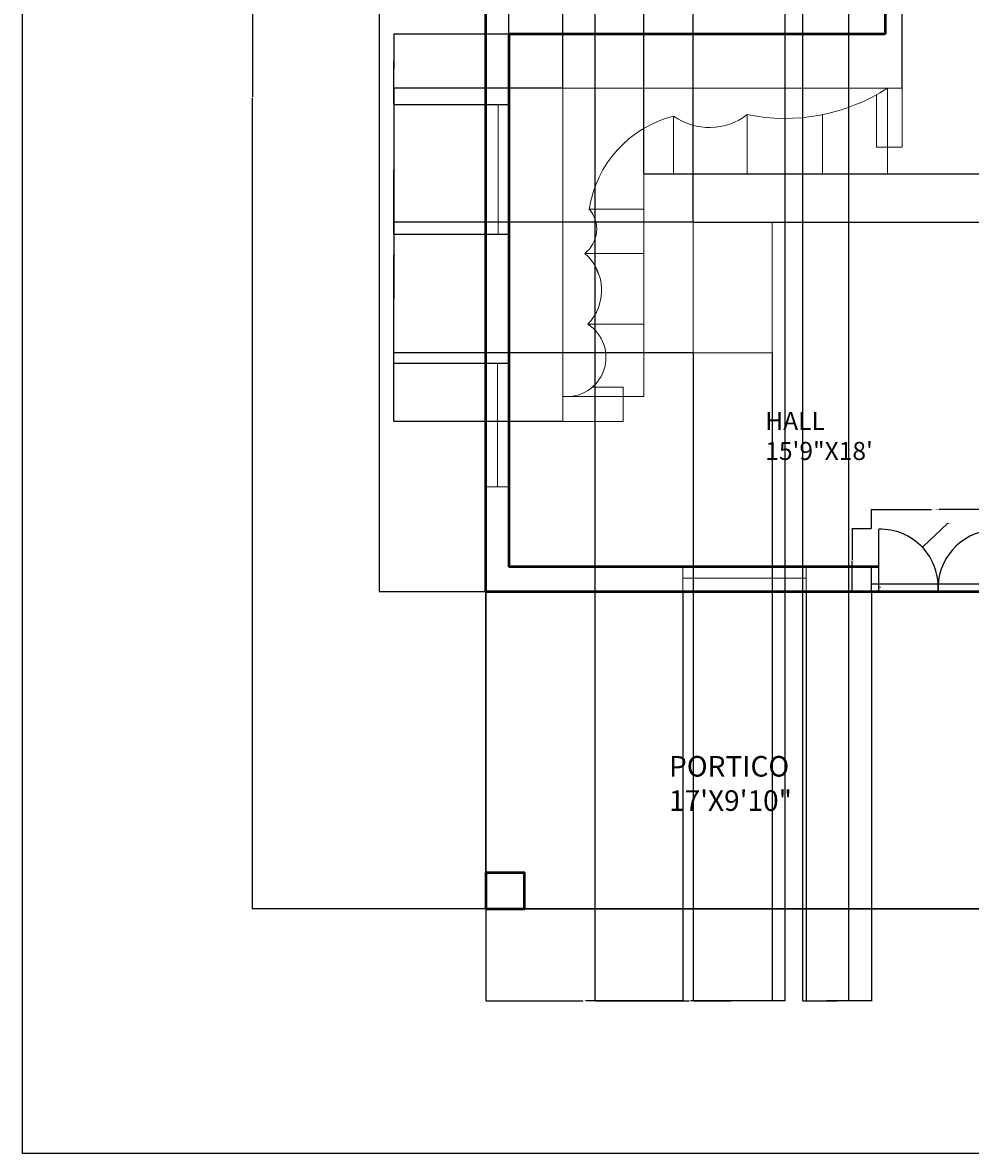
# Model space of a CAD drawing. Units: inches. Extents: x -177 to 2564, y -706 to 2548.
# Tile 1 of 4: x -177 to 192, y -706 to -266. Entities that reach past the tile are written whole.
import ezdxf

# ---------------------------------------------------------------- set-up
doc = ezdxf.new("R2010")
doc.units = ezdxf.units.IN
doc.header["$MEASUREMENT"] = 0
for name, color, linetype, lineweight in [('A-ANNO-DIMS', 2, 'Continuous', 18), ('A-ANNO-TTLB', 7, 'Continuous', 25), ('A-AREA-IDEN', 7, 'Continuous', 25), ('A-COLS', 7, 'Continuous', 50), ('A-DOOR', 3, 'Continuous', 25), ('A-FLOR-OTLN', 7, 'Continuous', 30), ('A-FURN', 8, 'Continuous', 18), ('A-GLAZ', 4, 'Continuous', 18), ('A-WALL', 7, 'Continuous', 50)]:
    doc.layers.add(name, color=color, linetype=linetype, lineweight=lineweight)
doc.styles.get("Standard").update_dxf_attribs({"font": 'arial.ttf'})
doc.dimstyles.get("Standard").update_dxf_attribs({"dimtxt": 0.18, "dimasz": 0.18, "dimexe": 0.18, "dimexo": 0.0625, "dimgap": 0.09, "dimtad": 0, "dimtih": 1, "dimtoh": 1, "dimdec": 0, "dimzin": 0, "dimdsep": 46, "dimlunit": 4, "dimtxsty": 'Standard', "dimcen": 0.09, "dimadec": 0, "dimazin": 0, "dimtfac": 1, "dimtdec": 0, "dimtofl": 0, "dimtmove": 0, "dimatfit": 3, "dimfxl": 1, "dimtolj": 1, "dimtzin": 0, "dimarcsym": 0})

# ---------------------------------------------------------------- blocks, each defined once
blk = doc.blocks.new('*D2')
at = {"layer": 'A-ANNO-DIMS', "color": 0, "lineweight": -2, "transparency": 16777216}
for p, q in [((3.41, 20.54), (-38, 20.54)), ((-37.82, 20.36), (-37.82, -233.15)), ((-37.82, -487.01), (-37.82, -233.51)), ((3.41, -487.19), (-38, -487.19))]:
    blk.add_line(p, q, dxfattribs=at)
at = {"layer": 'A-ANNO-DIMS', "color": 0, "transparency": 16777216}
for points in [[(-37.85, 20.36), (-37.79, 20.36), (-37.82, 20.54)], [(-37.85, -487.01), (-37.79, -487.01), (-37.82, -487.19)]]:
    blk.add_solid(points, dxfattribs=at)
at = {"layer": 'Defpoints', "color": 0, "transparency": 16777216}
for p in [(3.47, 20.54), (-37.82, -487.19), (3.47, -487.19)]:
    blk.add_point(p, dxfattribs=at)
at = {"layer": 'A-ANNO-DIMS', "color": 0, "transparency": 16777216, "insert": (-37.82, -233.33), "char_height": 0.18, "attachment_point": 5}
blk.add_mtext('\\A1;42\'-4"', dxfattribs=at)
blk = doc.blocks.new('*D3')
at = {"layer": 'A-ANNO-DIMS', "color": 0, "lineweight": -2, "transparency": 16777216}
for p, q in [((3.41, 20.54), (-87.46, 20.54)), ((-87.28, 20.36), (-87.28, -294.78)), ((-87.28, -610.28), (-87.28, -295.15)), ((3.41, -610.46), (-87.46, -610.46))]:
    blk.add_line(p, q, dxfattribs=at)
at = {"layer": 'A-ANNO-DIMS', "color": 0, "transparency": 16777216}
for points in [[(-87.31, 20.36), (-87.25, 20.36), (-87.28, 20.54)], [(-87.31, -610.28), (-87.25, -610.28), (-87.28, -610.46)]]:
    blk.add_solid(points, dxfattribs=at)
at = {"layer": 'Defpoints', "color": 0, "transparency": 16777216}
for p in [(3.47, 20.54), (-87.28, -610.46), (3.47, -610.46)]:
    blk.add_point(p, dxfattribs=at)
at = {"layer": 'A-ANNO-DIMS', "color": 0, "transparency": 16777216, "insert": (-87.28, -294.96), "char_height": 0.18, "attachment_point": 5}
blk.add_mtext('\\A1;52\'-7"', dxfattribs=at)
blk = doc.blocks.new('WIN-48')
for p, q in [((0, 0), (9, 0)), ((9, 0), (4.59, 0)), ((4.59, 0), (4.59, -48.06)), ((9, -48.06), (0, -48.06))]:
    blk.add_line(p, q)
blk = doc.blocks.new('DOOR-PAIR-44')
for p, q in [((0, 0), (0, 24.32)), ((44.01, 0), (44.01, 23.95)), ((-2.88, 0), (-2.88, 3.11)), ((-2.88, 3.11), (46.72, 3.11)), ((46.72, 0), (-2.88, 0)), ((-2.88, 0), (0, 0)), ((0, 0), (44.01, 0)), ((23.01, 0), (23.01, 3.55)), ((44.01, 0), (23.01, 0)), ((46.72, 0), (44.01, 0))]:
    blk.add_line(p, q)
for centre, radius, start, end in [((0.52, 1.77), 22.55, 355.4915, 91.326), ((45.7, 1.28), 22.73, 94.2755, 183.2347)]:
    blk.add_arc(centre, radius, start, end)
blk = doc.blocks.new('*D20')
at = {"layer": 'A-ANNO-DIMS', "color": 0, "lineweight": -2, "transparency": 16777216}
for p, q in [((153.41, -462.66), (153.41, -455.1)), ((153.59, -455.28), (176.76, -455.28)), ((202.83, -455.28), (179.66, -455.28)), ((203.01, -462.66), (203.01, -455.1))]:
    blk.add_line(p, q, dxfattribs=at)
at = {"layer": 'A-ANNO-DIMS', "color": 0, "transparency": 16777216}
for points in [[(153.59, -455.25), (153.59, -455.31), (153.41, -455.28)], [(202.83, -455.25), (202.83, -455.31), (203.01, -455.28)]]:
    blk.add_solid(points, dxfattribs=at)
at = {"layer": 'Defpoints', "color": 0, "transparency": 16777216}
for p in [(203.01, -455.28), (153.41, -462.72), (203.01, -462.72)]:
    blk.add_point(p, dxfattribs=at)
at = {"layer": 'A-ANNO-DIMS', "color": 0, "transparency": 16777216, "insert": (178.21, -455.28), "char_height": 0.18, "attachment_point": 5}
blk.add_mtext('\\A1;DOOR D3 4\'-1 1/2" TYP.', dxfattribs=at)
blk = doc.blocks.new('*D21')
at = {"layer": 'A-ANNO-DIMS', "color": 0, "lineweight": -2, "transparency": 16777216}
for p, q in [((153.34, -462.72), (145.79, -462.72)), ((145.97, -462.9), (145.97, -474.77)), ((145.97, -487.01), (145.97, -475.14)), ((153.34, -487.19), (145.79, -487.19))]:
    blk.add_line(p, q, dxfattribs=at)
at = {"layer": 'A-ANNO-DIMS', "color": 0, "transparency": 16777216}
for points in [[(145.94, -462.9), (146, -462.9), (145.97, -462.72)], [(145.94, -487.01), (146, -487.01), (145.97, -487.19)]]:
    blk.add_solid(points, dxfattribs=at)
at = {"layer": 'Defpoints', "color": 0, "transparency": 16777216}
for p in [(145.97, -462.72), (153.41, -462.72), (153.41, -487.19)]:
    blk.add_point(p, dxfattribs=at)
at = {"layer": 'A-ANNO-DIMS', "color": 0, "transparency": 16777216, "insert": (145.97, -474.95), "char_height": 0.18, "attachment_point": 5}
blk.add_mtext('\\A1;2\'-0 1/2" TYP.', dxfattribs=at)
blk = doc.blocks.new('*D22')
at = {"layer": 'A-ANNO-DIMS', "color": 0, "lineweight": -2, "transparency": 16777216}
for p, q in [((33.37, -291.35), (33.37, 71.74)), ((33.55, 71.56), (98.96, 71.56)), ((165.15, 71.56), (99.74, 71.56)), ((165.33, -291.35), (165.33, 71.74))]:
    blk.add_line(p, q, dxfattribs=at)
at = {"layer": 'A-ANNO-DIMS', "color": 0, "transparency": 16777216}
for points in [[(33.55, 71.59), (33.55, 71.53), (33.37, 71.56)], [(165.15, 71.59), (165.15, 71.53), (165.33, 71.56)]]:
    blk.add_solid(points, dxfattribs=at)
at = {"layer": 'Defpoints', "color": 0, "transparency": 16777216}
for p in [(165.33, 71.56), (33.37, -291.42), (165.33, -291.42)]:
    blk.add_point(p, dxfattribs=at)
at = {"layer": 'A-ANNO-DIMS', "color": 0, "transparency": 16777216, "insert": (99.35, 71.56), "char_height": 0.18, "attachment_point": 5}
blk.add_mtext('\\A1;11\'-0"', dxfattribs=at)
blk = doc.blocks.new('*D23')
at = {"layer": 'A-ANNO-DIMS', "color": 0, "lineweight": -2, "transparency": 16777216}
for p, q in [((33.31, -291.42), (-32.41, -291.42)), ((-32.23, -291.6), (-32.23, -356.01)), ((-32.23, -420.78), (-32.23, -356.37)), ((33.31, -420.96), (-32.41, -420.96))]:
    blk.add_line(p, q, dxfattribs=at)
at = {"layer": 'A-ANNO-DIMS', "color": 0, "transparency": 16777216}
for points in [[(-32.26, -291.6), (-32.2, -291.6), (-32.23, -291.42)], [(-32.26, -420.78), (-32.2, -420.78), (-32.23, -420.96)]]:
    blk.add_solid(points, dxfattribs=at)
at = {"layer": 'Defpoints', "color": 0, "transparency": 16777216}
for p in [(33.37, -291.42), (-32.23, -420.96), (33.37, -420.96)]:
    blk.add_point(p, dxfattribs=at)
at = {"layer": 'A-ANNO-DIMS', "color": 0, "transparency": 16777216, "insert": (-32.23, -356.19), "char_height": 0.18, "attachment_point": 5}
blk.add_mtext('\\A1;10\'-9 1/2"', dxfattribs=at)
blk = doc.blocks.new('*D24')
at = {"layer": 'A-ANNO-DIMS', "color": 0, "lineweight": -2, "transparency": 16777216}
for p, q in [((84.06, -394.33), (84.06, -646.34)), ((114.78, -394.33), (114.78, -646.34)), ((84.24, -646.16), (98.88, -646.16)), ((114.6, -646.16), (99.96, -646.16))]:
    blk.add_line(p, q, dxfattribs=at)
at = {"layer": 'A-ANNO-DIMS', "color": 0, "transparency": 16777216}
for points in [[(84.24, -646.13), (84.24, -646.19), (84.06, -646.16)], [(114.6, -646.13), (114.6, -646.19), (114.78, -646.16)]]:
    blk.add_solid(points, dxfattribs=at)
at = {"layer": 'Defpoints', "color": 0, "transparency": 16777216}
for p in [(84.06, -394.27), (114.78, -394.27), (114.78, -646.16)]:
    blk.add_point(p, dxfattribs=at)
at = {"layer": 'A-ANNO-DIMS', "color": 0, "transparency": 16777216, "insert": (99.42, -646.16), "char_height": 0.18, "attachment_point": 5}
blk.add_mtext('\\A1;2\'-6 1/2"', dxfattribs=at)
blk = doc.blocks.new('*D25')
at = {"layer": 'A-ANNO-DIMS', "color": 0, "lineweight": -2, "transparency": 16777216}
for p, q in [((84, -343.5), (-32.41, -343.5)), ((-32.23, -343.68), (-32.23, -368.7)), ((-32.23, -394.09), (-32.23, -369.07)), ((84, -394.27), (-32.41, -394.27))]:
    blk.add_line(p, q, dxfattribs=at)
at = {"layer": 'A-ANNO-DIMS', "color": 0, "transparency": 16777216}
for points in [[(-32.26, -343.68), (-32.2, -343.68), (-32.23, -343.5)], [(-32.26, -394.09), (-32.2, -394.09), (-32.23, -394.27)]]:
    blk.add_solid(points, dxfattribs=at)
at = {"layer": 'Defpoints', "color": 0, "transparency": 16777216}
for p in [(-32.23, -343.5), (84.06, -343.5), (84.06, -394.27)]:
    blk.add_point(p, dxfattribs=at)
at = {"layer": 'A-ANNO-DIMS', "color": 0, "transparency": 16777216, "insert": (-32.23, -368.89), "char_height": 0.18, "attachment_point": 5}
blk.add_mtext('\\A1;4\'-3"', dxfattribs=at)
blk = doc.blocks.new('*D26')
at = {"layer": 'A-ANNO-DIMS', "color": 0, "lineweight": -2, "transparency": 16777216}
for p, q in [((64.94, -324.62), (64.94, 71.74)), ((65.12, 71.56), (74.18, 71.56)), ((83.88, 71.56), (74.82, 71.56)), ((84.06, -343.44), (84.06, 71.74))]:
    blk.add_line(p, q, dxfattribs=at)
at = {"layer": 'A-ANNO-DIMS', "color": 0, "transparency": 16777216}
for points in [[(65.12, 71.59), (65.12, 71.53), (64.94, 71.56)], [(83.88, 71.59), (83.88, 71.53), (84.06, 71.56)]]:
    blk.add_solid(points, dxfattribs=at)
at = {"layer": 'Defpoints', "color": 0, "transparency": 16777216}
for p in [(84.06, 71.56), (64.94, -324.69), (84.06, -343.5)]:
    blk.add_point(p, dxfattribs=at)
at = {"layer": 'A-ANNO-DIMS', "color": 0, "transparency": 16777216, "insert": (74.5, 71.56), "char_height": 0.18, "attachment_point": 5}
blk.add_mtext('\\A1;1\'-7"', dxfattribs=at)
blk = doc.blocks.new('*D27')
at = {"layer": 'A-ANNO-DIMS', "color": 0, "lineweight": -2, "transparency": 16777216}
for p, q in [((65.01, -324.69), (417.35, -324.69)), ((417.17, -324.87), (417.17, -333.91)), ((417.17, -343.32), (417.17, -334.27)), ((84.12, -343.5), (417.35, -343.5))]:
    blk.add_line(p, q, dxfattribs=at)
at = {"layer": 'A-ANNO-DIMS', "color": 0, "transparency": 16777216}
for points in [[(417.14, -324.87), (417.2, -324.87), (417.17, -324.69)], [(417.14, -343.32), (417.2, -343.32), (417.17, -343.5)]]:
    blk.add_solid(points, dxfattribs=at)
at = {"layer": 'Defpoints', "color": 0, "transparency": 16777216}
for p in [(64.94, -324.69), (84.06, -343.5), (417.17, -343.5)]:
    blk.add_point(p, dxfattribs=at)
at = {"layer": 'A-ANNO-DIMS', "color": 0, "transparency": 16777216, "insert": (417.17, -334.09), "char_height": 0.18, "attachment_point": 5}
blk.add_mtext('\\A1;1\'-7"', dxfattribs=at)
blk = doc.blocks.new('*D28')
at = {"layer": 'A-ANNO-DIMS', "color": 0, "lineweight": -2, "transparency": 16777216}
for p, q in [((12.47, -270.4), (12.47, 71.74)), ((12.65, 71.56), (22.6, 71.56)), ((33.19, 71.56), (23.24, 71.56)), ((33.37, -291.35), (33.37, 71.74))]:
    blk.add_line(p, q, dxfattribs=at)
at = {"layer": 'A-ANNO-DIMS', "color": 0, "transparency": 16777216}
for points in [[(12.65, 71.59), (12.65, 71.53), (12.47, 71.56)], [(33.19, 71.59), (33.19, 71.53), (33.37, 71.56)]]:
    blk.add_solid(points, dxfattribs=at)
at = {"layer": 'Defpoints', "color": 0, "transparency": 16777216}
for p in [(33.37, 71.56), (12.47, -270.46), (33.37, -291.42)]:
    blk.add_point(p, dxfattribs=at)
at = {"layer": 'A-ANNO-DIMS', "color": 0, "transparency": 16777216, "insert": (22.92, 71.56), "char_height": 0.18, "attachment_point": 5}
blk.add_mtext('\\A1;1\'-9"', dxfattribs=at)
blk = doc.blocks.new('*D29')
at = {"layer": 'A-ANNO-DIMS', "color": 0, "lineweight": -2, "transparency": 16777216}
for p, q in [((12.41, -270.46), (-32.41, -270.46)), ((-32.23, -270.64), (-32.23, -280.76)), ((-32.23, -291.24), (-32.23, -281.12)), ((33.31, -291.42), (-32.41, -291.42))]:
    blk.add_line(p, q, dxfattribs=at)
at = {"layer": 'A-ANNO-DIMS', "color": 0, "transparency": 16777216}
for points in [[(-32.26, -270.64), (-32.2, -270.64), (-32.23, -270.46)], [(-32.26, -291.24), (-32.2, -291.24), (-32.23, -291.42)]]:
    blk.add_solid(points, dxfattribs=at)
at = {"layer": 'Defpoints', "color": 0, "transparency": 16777216}
for p in [(12.47, -270.46), (-32.23, -291.42), (33.37, -291.42)]:
    blk.add_point(p, dxfattribs=at)
at = {"layer": 'A-ANNO-DIMS', "color": 0, "transparency": 16777216, "insert": (-32.23, -280.94), "char_height": 0.18, "attachment_point": 5}
blk.add_mtext('\\A1;1\'-9"', dxfattribs=at)
blk = doc.blocks.new('*D32')
at = {"layer": 'A-ANNO-DIMS', "color": 0, "lineweight": -2, "transparency": 16777216}
for p, q in [((45.91, -17.28), (45.91, -646.34)), ((119.76, -17.28), (119.76, -646.34)), ((46.09, -646.16), (82.5, -646.16)), ((119.58, -646.16), (83.16, -646.16))]:
    blk.add_line(p, q, dxfattribs=at)
at = {"layer": 'A-ANNO-DIMS', "color": 0, "transparency": 16777216}
for points in [[(46.09, -646.13), (46.09, -646.19), (45.91, -646.16)], [(119.58, -646.13), (119.58, -646.19), (119.76, -646.16)]]:
    blk.add_solid(points, dxfattribs=at)
at = {"layer": 'Defpoints', "color": 0, "transparency": 16777216}
for p in [(45.91, -17.21), (119.76, -17.21), (119.76, -646.16)]:
    blk.add_point(p, dxfattribs=at)
at = {"layer": 'A-ANNO-DIMS', "color": 0, "transparency": 16777216, "insert": (82.83, -646.16), "char_height": 0.18, "attachment_point": 5}
blk.add_mtext('\\A1;6\'-2"', dxfattribs=at)
blk = doc.blocks.new('*D33')
at = {"layer": 'A-ANNO-DIMS', "color": 0, "lineweight": -2, "transparency": 16777216}
for p, q in [((126.64, -61.62), (126.64, -646.34)), ((144.47, -61.62), (144.47, -646.34)), ((126.82, -646.16), (135.24, -646.16)), ((144.29, -646.16), (135.88, -646.16))]:
    blk.add_line(p, q, dxfattribs=at)
at = {"layer": 'A-ANNO-DIMS', "color": 0, "transparency": 16777216}
for points in [[(126.82, -646.13), (126.82, -646.19), (126.64, -646.16)], [(144.29, -646.13), (144.29, -646.19), (144.47, -646.16)]]:
    blk.add_solid(points, dxfattribs=at)
at = {"layer": 'Defpoints', "color": 0, "transparency": 16777216}
for p in [(126.64, -61.56), (144.47, -61.56), (144.47, -646.16)]:
    blk.add_point(p, dxfattribs=at)
at = {"layer": 'A-ANNO-DIMS', "color": 0, "transparency": 16777216, "insert": (135.56, -646.16), "char_height": 0.18, "attachment_point": 5}
blk.add_mtext('\\A1;1\'-6"', dxfattribs=at)
blk = doc.blocks.new('*D38')
at = {"layer": 'A-ANNO-DIMS', "color": 0, "lineweight": -2, "transparency": 16777216}
for p, q in [((3.47, -487.25), (3.47, -646.34)), ((80.08, -487.25), (80.08, -646.34)), ((3.65, -646.16), (41.24, -646.16)), ((79.9, -646.16), (42.32, -646.16))]:
    blk.add_line(p, q, dxfattribs=at)
at = {"layer": 'A-ANNO-DIMS', "color": 0, "transparency": 16777216}
for points in [[(3.65, -646.13), (3.65, -646.19), (3.47, -646.16)], [(79.9, -646.13), (79.9, -646.19), (80.08, -646.16)]]:
    blk.add_solid(points, dxfattribs=at)
at = {"layer": 'Defpoints', "color": 0, "transparency": 16777216}
for p in [(3.47, -487.19), (80.08, -487.19), (80.08, -646.16)]:
    blk.add_point(p, dxfattribs=at)
at = {"layer": 'A-ANNO-DIMS', "color": 0, "transparency": 16777216, "insert": (41.78, -646.16), "char_height": 0.18, "attachment_point": 5}
blk.add_mtext('\\A1;6\'-4 1/2"', dxfattribs=at)
blk = doc.blocks.new('*D39')
at = {"layer": 'A-ANNO-DIMS', "color": 0, "lineweight": -2, "transparency": 16777216}
for p, q in [((128.08, -487.25), (128.08, -646.34)), ((153.41, -487.25), (153.41, -646.34)), ((128.26, -646.16), (140.2, -646.16)), ((153.23, -646.16), (141.28, -646.16))]:
    blk.add_line(p, q, dxfattribs=at)
at = {"layer": 'A-ANNO-DIMS', "color": 0, "transparency": 16777216}
for points in [[(128.26, -646.13), (128.26, -646.19), (128.08, -646.16)], [(153.23, -646.13), (153.23, -646.19), (153.41, -646.16)]]:
    blk.add_solid(points, dxfattribs=at)
at = {"layer": 'Defpoints', "color": 0, "transparency": 16777216}
for p in [(128.08, -487.19), (153.41, -487.19), (153.41, -646.16)]:
    blk.add_point(p, dxfattribs=at)
at = {"layer": 'A-ANNO-DIMS', "color": 0, "transparency": 16777216, "insert": (140.74, -646.16), "char_height": 0.18, "attachment_point": 5}
blk.add_mtext('\\A1;2\'-1 1/2"', dxfattribs=at)
blk = doc.blocks.new('*D56')
at = {"layer": 'A-ANNO-DIMS', "color": 0, "lineweight": -2, "transparency": 16777216}
for p, q in [((12.41, -270.46), (-32.41, -270.46)), ((-32.23, -270.64), (-32.23, -284)), ((-32.23, -297.73), (-32.23, -284.37)), ((12.41, -297.91), (-32.41, -297.91))]:
    blk.add_line(p, q, dxfattribs=at)
at = {"layer": 'A-ANNO-DIMS', "color": 0, "transparency": 16777216}
for points in [[(-32.26, -270.64), (-32.2, -270.64), (-32.23, -270.46)], [(-32.26, -297.73), (-32.2, -297.73), (-32.23, -297.91)]]:
    blk.add_solid(points, dxfattribs=at)
at = {"layer": 'Defpoints', "color": 0, "transparency": 16777216}
for p in [(12.47, -270.46), (-32.23, -297.91), (12.47, -297.91)]:
    blk.add_point(p, dxfattribs=at)
at = {"layer": 'A-ANNO-DIMS', "color": 0, "transparency": 16777216, "insert": (-32.23, -284.19), "char_height": 0.18, "attachment_point": 5}
blk.add_mtext('\\A1;2\'-3 1/2"', dxfattribs=at)
blk = doc.blocks.new('*D57')
at = {"layer": 'A-ANNO-DIMS', "color": 0, "lineweight": -2, "transparency": 16777216}
for p, q in [((12.41, -297.91), (-32.41, -297.91)), ((-32.23, -298.09), (-32.23, -322.91)), ((-32.23, -348.09), (-32.23, -323.27)), ((12.41, -348.27), (-32.41, -348.27))]:
    blk.add_line(p, q, dxfattribs=at)
at = {"layer": 'A-ANNO-DIMS', "color": 0, "transparency": 16777216}
for points in [[(-32.26, -298.09), (-32.2, -298.09), (-32.23, -297.91)], [(-32.26, -348.09), (-32.2, -348.09), (-32.23, -348.27)]]:
    blk.add_solid(points, dxfattribs=at)
at = {"layer": 'Defpoints', "color": 0, "transparency": 16777216}
for p in [(12.47, -297.91), (-32.23, -348.27), (12.47, -348.27)]:
    blk.add_point(p, dxfattribs=at)
at = {"layer": 'A-ANNO-DIMS', "color": 0, "transparency": 16777216, "insert": (-32.23, -323.09), "char_height": 0.18, "attachment_point": 5}
blk.add_mtext('\\A1;4\'-2 1/2"', dxfattribs=at)
blk = doc.blocks.new('*D58')
at = {"layer": 'A-ANNO-DIMS', "color": 0, "lineweight": -2, "transparency": 16777216}
for p, q in [((12.41, -348.27), (-32.41, -348.27)), ((-32.23, -348.45), (-32.23, -373.16)), ((-32.23, -398.23), (-32.23, -373.52)), ((12.41, -398.41), (-32.41, -398.41))]:
    blk.add_line(p, q, dxfattribs=at)
at = {"layer": 'A-ANNO-DIMS', "color": 0, "transparency": 16777216}
for points in [[(-32.26, -348.45), (-32.2, -348.45), (-32.23, -348.27)], [(-32.26, -398.23), (-32.2, -398.23), (-32.23, -398.41)]]:
    blk.add_solid(points, dxfattribs=at)
at = {"layer": 'Defpoints', "color": 0, "transparency": 16777216}
for p in [(12.47, -348.27), (-32.23, -398.41), (12.47, -398.41)]:
    blk.add_point(p, dxfattribs=at)
at = {"layer": 'A-ANNO-DIMS', "color": 0, "transparency": 16777216, "insert": (-32.23, -373.34), "char_height": 0.18, "attachment_point": 5}
blk.add_mtext('\\A1;4\'-2"', dxfattribs=at)
blk = doc.blocks.new('*D65')
at = {"layer": 'A-ANNO-DIMS', "color": 0, "lineweight": -2, "transparency": 16777216}
for p, q in [((183.03, -460.62), (173.33, -469.79)), ((183.21, -460.62), (183.03, -460.62)), ((156.72, -485.41), (156.9, -485.41)), ((156.81, -485.5), (156.81, -485.32))]:
    blk.add_line(p, q, dxfattribs=at)
at = {"layer": 'A-ANNO-DIMS', "color": 0, "transparency": 16777216}
blk.add_solid([(173.31, -469.77), (173.35, -469.81), (173.2, -469.92)], dxfattribs=at)
at = {"layer": 'Defpoints', "color": 0, "transparency": 16777216}
for p in [(173.2, -469.92), (156.81, -485.41)]:
    blk.add_point(p, dxfattribs=at)
at = {"layer": 'A-ANNO-DIMS', "color": 0, "transparency": 16777216, "insert": (184.1, -460.62), "char_height": 0.18, "attachment_point": 5}
blk.add_mtext('\\A1;2X R1\'-10 1/2"', dxfattribs=at)

msp = doc.modelspace()

# ---------------------------------------------------------------- linework, layer by layer
at = {"layer": 'A-ANNO-TTLB'}
msp.add_lwpolyline([(-176.6, 185.58), (523.32, 185.58), (523.32, -705.52), (-176.6, -705.52)], close=True, dxfattribs=at)
at = {"layer": 'A-COLS'}
msp.add_lwpolyline([(3.47, -610.46), (18.48, -610.46), (18.48, -596.46), (3.47, -596.46)], close=True, dxfattribs=at)
at = {"layer": 'A-DOOR'}
msp.add_line((153.41, -487.19), (153.41, -477.46), dxfattribs=at)
at = {"layer": 'A-FLOR-OTLN'}
for p, q in [((3.47, -601.46), (3.47, -487.19)), ((3.47, -610.46), (3.47, -601.46)), ((228.47, -610.46), (3.47, -610.46))]:
    msp.add_line(p, q, dxfattribs=at)
at = {"layer": 'A-FURN'}
for p, q in [((33.37, -291.42), (159.67, -291.42)), ((33.37, -411.3), (33.37, -291.42)), ((155.39, -314.44), (155.39, -293.99)), ((159.67, -291.42), (159.67, -324.69)), ((159.67, -291.42), (165.33, -291.42)), ((165.33, -291.42), (165.33, -314.44)), ((76.43, -324.69), (76.43, -302.31)), ((105.13, -324.69), (105.13, -301.74)), ((134.41, -324.69), (134.41, -301.74)), ((165.33, -314.44), (155.39, -314.44)), ((159.67, -324.69), (64.94, -324.69)), ((64.94, -324.69), (64.94, -411.3)), ((105.13, -324.69), (76.43, -324.69)), ((134.41, -324.69), (105.13, -324.69)), ((159.67, -324.69), (134.41, -324.69)), ((64.94, -338.45), (43.7, -338.45)), ((64.94, -355.66), (64.94, -338.45)), ((64.94, -355.66), (41.98, -355.66)), ((64.94, -383.2), (64.94, -355.66)), ((64.94, -383.2), (43.13, -383.2)), ((64.94, -411.3), (64.94, -383.2)), ((56.92, -407.71), (44.83, -407.71)), ((56.92, -420.96), (56.92, -407.71)), ((64.94, -411.3), (33.37, -411.3)), ((33.37, -411.3), (33.37, -420.96)), ((33.37, -420.96), (56.92, -420.96))]:
    msp.add_line(p, q, dxfattribs=at)
msp.add_lwpolyline([(84.06, -343.5), (114.78, -343.5), (114.78, -394.27), (84.06, -394.27)], close=True, dxfattribs=at)
for centre, radius, start, end in [((119.77, -229.86), 73.36, 258.488, 302.952), ((87.39, -345.13), 44.19, 104.3618, 171.3148), ((90.39, -282.55), 24.2, 234.764, 307.5256), ((34.63, -346.24), 11.95, 307.9515, 40.6177), ((29.44, -369.98), 19.03, 315.9974, 48.7785), ((87.39, -345.13), 44.19, 200.4463, 205.9744), ((34.89, -396.09), 15.3, 264.277, 57.4256)]:
    msp.add_arc(centre, radius, start, end, dxfattribs=at)
at = {"layer": 'A-GLAZ'}
for p, q in [((12.47, -297.91), (3.47, -297.91)), ((3.47, -297.91), (3.47, -348.27)), ((8.31, -348.27), (8.31, -297.91)), ((3.47, -348.27), (12.47, -348.27)), ((12.47, -348.27), (8.31, -348.27)), ((12.47, -348.27), (12.47, -348.27)), ((3.47, -446.47), (3.47, -398.41)), ((80.08, -487.19), (80.08, -477.46)), ((80.08, -477.46), (80.08, -481.92)), ((128.08, -477.46), (128.08, -487.19)), ((80.08, -481.92), (128.08, -481.92)), ((128.08, -487.19), (80.08, -487.19))]:
    msp.add_line(p, q, dxfattribs=at)
at = {"layer": 'A-WALL'}
for p, q in [((3.47, -483.46), (3.47, 20.54)), ((158.78, -261.46), (158.78, -270.46)), ((158.78, -270.46), (12.47, -270.46)), ((12.47, -270.46), (12.47, -297.91)), ((12.47, -270.46), (12.47, -477.46)), ((156.29, -477.46), (12.47, -477.46)), ((153.41, -477.46), (128.08, -477.46)), ((3.47, -487.19), (3.47, -483.46)), ((219.47, -487.19), (3.47, -487.19))]:
    msp.add_line(p, q, dxfattribs=at)

# ---------------------------------------------------------------- block references
at = {"layer": 'A-DOOR'}
msp.add_blockref('DOOR-PAIR-44', (156.29, -487.19), dxfattribs=at)
at = {"layer": 'A-GLAZ'}
msp.add_blockref('WIN-48', (3.47, -398.41), dxfattribs=at)

# ---------------------------------------------------------------- texts
at = {"layer": 'A-AREA-IDEN', "insert": (112.13, -417.3), "char_height": 7, "attachment_point": 1}
msp.add_mtext_dynamic_manual_height_columns('HALL\\P15\'9"X18\'', width=0.5909, gutter_width=1, heights=[0], dxfattribs=at)
at = {"layer": 'A-AREA-IDEN', "insert": (74.71, -551.05), "char_height": 8, "attachment_point": 1}
msp.add_mtext('PORTICO\\P17\'X9\'10"', dxfattribs=at)

# ---------------------------------------------------------------- dimensions: what is measured, and where the dimension line sits
at = {"layer": 'A-ANNO-DIMS'}
for base, p1, p2, picture, middle in [((33.37, 71.56), (12.47, -270.46), (33.37, -291.42), '*D28', (22.92, 71.56)), ((165.33, 71.56), (33.37, -291.42), (165.33, -291.42), '*D22', (99.35, 71.56)), ((84.06, 71.56), (64.94, -324.69), (84.06, -343.5), '*D26', (74.5, 71.56)), ((119.7563, -646.1645), (45.9113, -17.2143), (119.7563, -17.2143), '*D32', (82.8338, -646.1645)), ((144.47, -646.16), (126.64, -61.56), (144.47, -61.56), '*D33', (135.56, -646.16)), ((114.78, -646.16), (84.06, -394.27), (114.78, -394.27), '*D24', (99.42, -646.16)), ((80.08, -646.16), (3.47, -487.19), (80.08, -487.19), '*D38', (41.78, -646.16)), ((153.41, -646.16), (128.08, -487.19), (153.41, -487.19), '*D39', (140.74, -646.16))]:
    dim = msp.add_linear_dim(base=base, p1=p1, p2=p2, dimstyle='Standard', override={"dimdec": 1, "dimlfac": 1, "dimrnd": 0, "dimzin": 1, "dimdsep": 46, "dimlunit": 4, "dimfrac": 2}, dxfattribs=at)
    dim.commit()
    dim.dimension.update_dxf_attribs({"geometry": picture, "text_midpoint": middle})
for base, p1, p2, override, picture, middle in [((-87.28, -610.46), (3.47, 20.54), (3.47, -610.46), {"dimclrd": 0, "dimclre": 0, "dimclrt": 0}, '*D3', (-87.28, -294.96)), ((-37.82, -487.19), (3.47, 20.54), (3.47, -487.19), {"dimclrd": 0, "dimclre": 0, "dimclrt": 0}, '*D2', (-37.82, -233.33)), ((-32.2267, -297.9061), (12.4733, -270.4645), (12.4733, -297.9061), {"dimdec": 1, "dimlfac": 1, "dimrnd": 0, "dimzin": 1, "dimdsep": 46, "dimlunit": 4, "dimfrac": 2}, '*D56', (-32.2267, -284.1853)), ((-32.23, -291.42), (12.47, -270.46), (33.37, -291.42), {"dimdec": 1, "dimlfac": 1, "dimrnd": 0, "dimzin": 1, "dimdsep": 46, "dimlunit": 4, "dimfrac": 2}, '*D29', (-32.23, -280.94)), ((-32.23, -420.96), (33.37, -291.42), (33.37, -420.96), {"dimdec": 1, "dimlfac": 1, "dimrnd": 0, "dimzin": 1, "dimdsep": 46, "dimlunit": 4, "dimfrac": 2}, '*D23', (-32.23, -356.19)), ((-32.23, -348.27), (12.47, -297.91), (12.47, -348.27), {"dimdec": 1, "dimlfac": 1, "dimrnd": 0, "dimzin": 1, "dimdsep": 46, "dimlunit": 4, "dimfrac": 2}, '*D57', (-32.23, -323.09)), ((417.17, -343.5), (64.94, -324.69), (84.06, -343.5), {"dimdec": 1, "dimlfac": 1, "dimrnd": 0, "dimzin": 1, "dimdsep": 46, "dimlunit": 4, "dimfrac": 2}, '*D27', (417.17, -334.09)), ((-32.23, -343.5), (84.06, -394.27), (84.06, -343.5), {"dimdec": 1, "dimlfac": 1, "dimrnd": 0, "dimzin": 1, "dimdsep": 46, "dimlunit": 4, "dimfrac": 2}, '*D25', (-32.23, -368.89)), ((-32.23, -398.41), (12.47, -348.27), (12.47, -398.41), {"dimdec": 1, "dimlfac": 1, "dimrnd": 0, "dimzin": 1, "dimdsep": 46, "dimlunit": 4, "dimfrac": 2}, '*D58', (-32.23, -373.34))]:
    dim = msp.add_linear_dim(base=base, p1=p1, p2=p2, angle=90, dimstyle='Standard', override=override, dxfattribs=at)
    dim.commit()
    dim.dimension.update_dxf_attribs({"geometry": picture, "text_midpoint": middle})
dim = msp.add_linear_dim(base=(203.01, -455.28), p1=(153.41, -462.72), p2=(203.01, -462.72), text='DOOR D3 <> TYP.', dimstyle='Standard', override={"dimdec": 1, "dimlfac": 1, "dimrnd": 0, "dimzin": 1, "dimdsep": 46, "dimlunit": 4, "dimfrac": 2}, dxfattribs=at)
dim.commit()
dim.dimension.update_dxf_attribs({"geometry": '*D20', "text_midpoint": (178.21, -455.28)})
dim = msp.add_radius_dim(center=(156.81, -485.41), mpoint=(173.2, -469.92), text='2X <>', dimstyle='Standard', override={"dimdec": 1, "dimlfac": 1, "dimrnd": 0, "dimzin": 1, "dimdsep": 46, "dimlunit": 4, "dimfrac": 2}, dxfattribs=at)
dim.commit()
dim.dimension.update_dxf_attribs({"geometry": '*D65', "text_midpoint": (184.1, -460.62), "dimtype": 164})
dim = msp.add_linear_dim(base=(145.97, -462.72), p1=(153.41, -487.19), p2=(153.41, -462.72), angle=90, text='<> TYP.', dimstyle='Standard', override={"dimdec": 1, "dimlfac": 1, "dimrnd": 0, "dimzin": 1, "dimdsep": 46, "dimlunit": 4, "dimfrac": 2}, dxfattribs=at)
dim.commit()
dim.dimension.update_dxf_attribs({"geometry": '*D21', "text_midpoint": (145.97, -474.95)})

doc.saveas('drawing.dxf')
